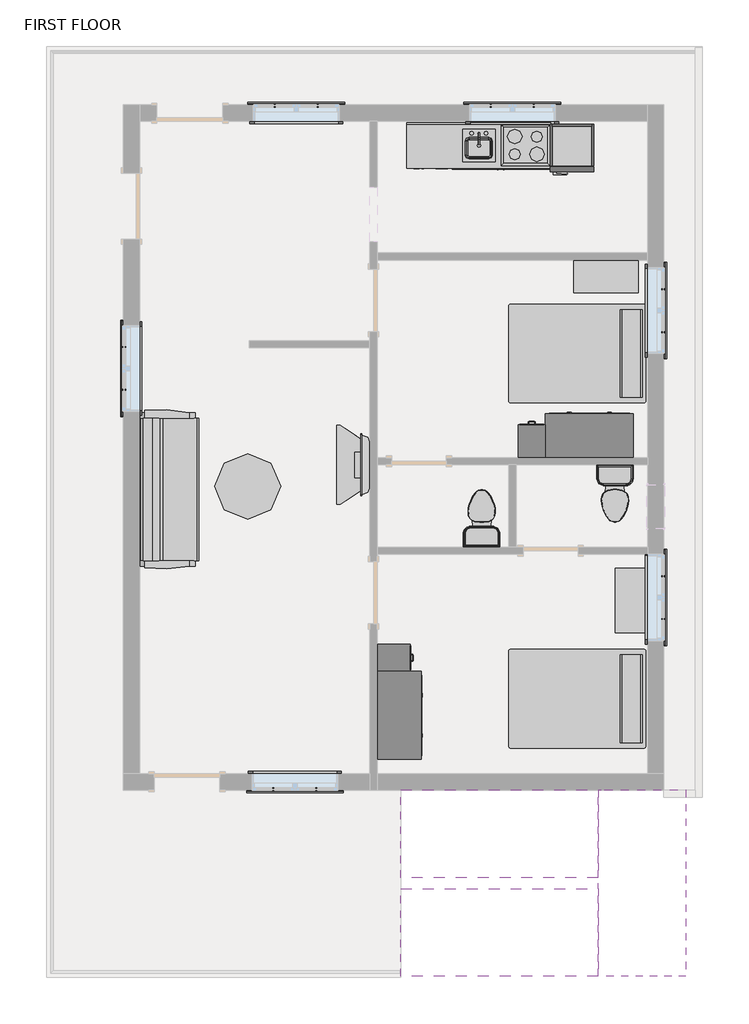
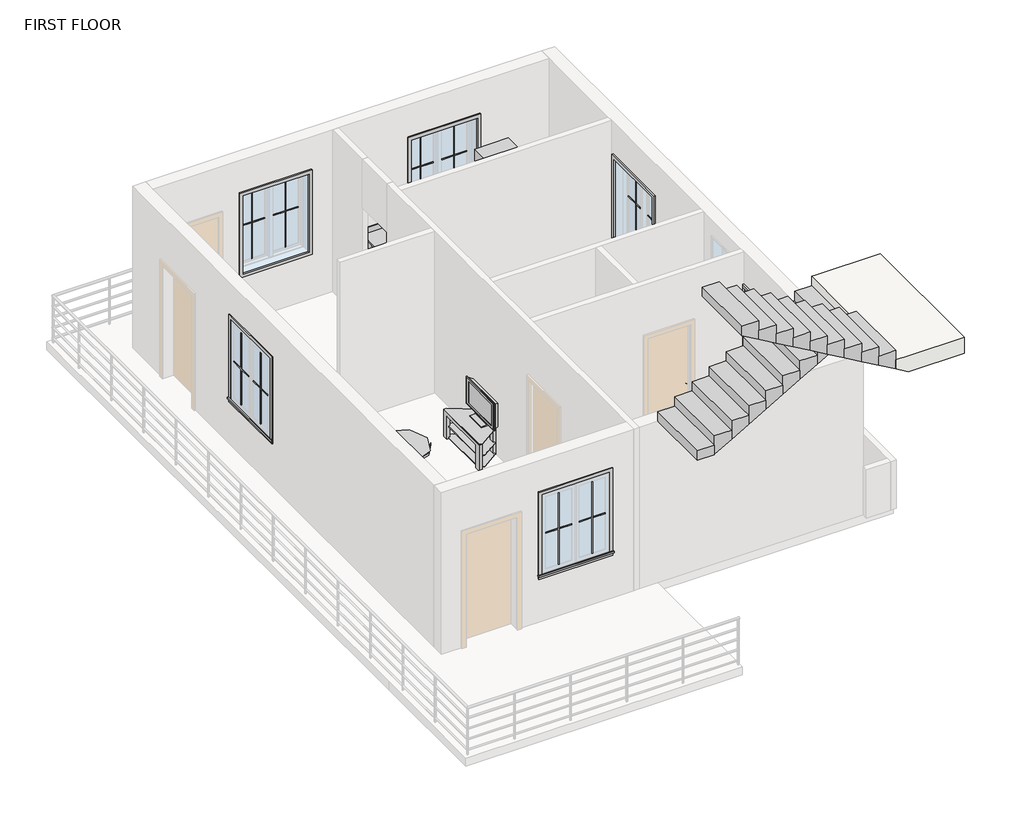
# One storey, part 3 of 3: 28 proxies, 13 furniture elements, 3 flow terminals, 2 stair flights, 1 slab.
"""IFC4 building model written with IfcOpenShell, lengths in millimetres."""

from ifc_helpers import new_model, si_unit, origin, place, context, project, spatial, faceted_brep, transform, mapped, element, save
from components import m_cook_top_4_unit2_0615_x_500mm_c91639ce, m_dishwasher_610_x_610_x_875mm_75336c20, m_kitchenette_medium_m_kitchenette_medium_71e50c56, m_muntin_pattern_2x2_m_muntin_pattern_2x2_d4676b39, m_muntin_pattern_2x2_m_muntin_pattern_2x2_dce6eb8c, m_refrigerator_600_x_660mm_0a899b9c, m_trim_window_exterior_flat_with_sill_a970d7bf, m_trim_window_interior_flat_picture_frame_5bf35ee4, m_sink_kitchen_island_450_x_450mm_f6c2c534, m_toilet_domestic_3d_m_toilet_domestic_3d_ba6479b0, m_toilet_domestic_3d_m_toilet_domestic_3d_1a010dbe, furniture_dc210597, furniture_0810mm_51289c3c, m_bed_standard_1372_x_1905mm_double_64e02cd7, m_cabinet_file_5_drawer_0380_x_0457mm_21dee09a, m_counter_top_w_sink_hole_600mm_depth_2c7d9717, m_dresser_1220_x_1830_x_0610mm_75a9f440, m_furniture_system_storage_cabinet_2_vertical_file_900_x_450_def3fd80, m_sofa_pensi_2134mm_538a523a, m_table_dining_round_0915mm_diameter_394c0b6d

model = new_model("IFC4")

# Units and contexts
model_context = context("Model", 3, world=origin())
ifc_project = project(units=[si_unit("LENGTHUNIT", "METRE", prefix="MILLI")], contexts=[model_context])

# Site, building, storey
site = spatial("IfcSite", under=ifc_project)
building = spatial("IfcBuilding", under=site)
storey = spatial("IfcBuildingStorey", under=building, Name="FIRST FLOOR", Elevation=3200.4)

# Proxies
placement = place(None, origin())
m_cook_top_4_unit2_0615_x_500mm_shape = m_cook_top_4_unit2_0615_x_500mm_c91639ce(model_context)
element("IfcBuildingElementProxy", 1, Name="M_Cook Top-4 Unit2 : 0615 x 500mm", ObjectType="M_Cook Top-4 Unit2 : 0615 x 500mm", at=placement, inside=storey, context=model_context, shape_type="MappedRepresentation", body=[
    mapped(m_cook_top_4_unit2_0615_x_500mm_shape, transform((1952.0701854, 4546.4851347, 3215.4), x_axis=(-1.0, 0.0, 0.0), y_axis=(0.0, -1.0, 0.0), z_axis=(0.0, 0.0, 1.0))),
])
m_dishwasher_610_x_610_x_875mm_shape = m_dishwasher_610_x_610_x_875mm_75336c20(model_context)
element("IfcBuildingElementProxy", 2, Name="M_Dishwasher : 610 x 610 x 875mm", ObjectType="M_Dishwasher : 610 x 610 x 875mm", at=placement, inside=storey, context=model_context, shape_type="MappedRepresentation", body=[
    mapped(m_dishwasher_610_x_610_x_875mm_shape, transform((987.0876539, 4289.8355699, 3200.4), x_axis=(-1.0, 0.0, 0.0), y_axis=(0.0, -1.0, 0.0), z_axis=(0.0, 0.0, 1.0))),
])
m_kitchenette_medium_m_kitchenette_medium_shape = m_kitchenette_medium_m_kitchenette_medium_71e50c56(model_context)
element("IfcBuildingElementProxy", 3, Name="M_Kitchenette - Medium : M_Kitchenette - Medium", ObjectType="M_Kitchenette - Medium : M_Kitchenette - Medium", at=placement, inside=storey, context=model_context, shape_type="MappedRepresentation", body=[
    mapped(m_kitchenette_medium_m_kitchenette_medium_shape, transform((1623.3078903, 4861.4851347, 3200.4), x_axis=(-1.0, 0.0, 0.0), y_axis=(0.0, -1.0, 0.0), z_axis=(0.0, 0.0, 1.0))),
])
m_muntin_pattern_2x2_m_muntin_pattern_2x2_shape = m_muntin_pattern_2x2_m_muntin_pattern_2x2_d4676b39(model_context)
element("IfcBuildingElementProxy", 4, Name="M_Muntin Pattern_2x2 : M_Muntin Pattern_2x2", ObjectType="M_Muntin Pattern_2x2 : M_Muntin Pattern_2x2", at=placement, inside=storey, context=model_context, shape_type="MappedRepresentation", body=[
    mapped(m_muntin_pattern_2x2_m_muntin_pattern_2x2_shape, transform((1466.9330952, 5099.6101347, 4170.25), x_axis=(1.0, 0.0, 0.0), y_axis=(0.0, 1.0, 0.0), z_axis=(0.0, 0.0, 1.0))),
])
element("IfcBuildingElementProxy", 5, Name="M_Muntin Pattern_2x2 : M_Muntin Pattern_2x2", ObjectType="M_Muntin Pattern_2x2 : M_Muntin Pattern_2x2", at=placement, inside=storey, context=model_context, shape_type="MappedRepresentation", body=[
    mapped(m_muntin_pattern_2x2_m_muntin_pattern_2x2_shape, transform((3864.0205952, 2548.5476347, 4170.25), x_axis=(0.0, -1.0, 0.0), y_axis=(1.0, 0.0, 0.0), z_axis=(0.0, 0.0, 1.0))),
])
element("IfcBuildingElementProxy", 6, Name="M_Muntin Pattern_2x2 : M_Muntin Pattern_2x2", ObjectType="M_Muntin Pattern_2x2 : M_Muntin Pattern_2x2", at=placement, inside=storey, context=model_context, shape_type="MappedRepresentation", body=[
    mapped(m_muntin_pattern_2x2_m_muntin_pattern_2x2_shape, transform((3864.0205952, -1440.8523653, 4170.25), x_axis=(0.0, -1.0, 0.0), y_axis=(1.0, 0.0, 0.0), z_axis=(0.0, 0.0, 1.0))),
])
element("IfcBuildingElementProxy", 7, Name="M_Muntin Pattern_2x2 : M_Muntin Pattern_2x2", ObjectType="M_Muntin Pattern_2x2 : M_Muntin Pattern_2x2", at=placement, inside=storey, context=model_context, shape_type="MappedRepresentation", body=[
    mapped(m_muntin_pattern_2x2_m_muntin_pattern_2x2_shape, transform((-3635.3294048, 1147.1226347, 4170.25), x_axis=(0.0, 1.0, 0.0), y_axis=(-1.0, 0.0, 0.0), z_axis=(0.0, 0.0, 1.0))),
])
element("IfcBuildingElementProxy", 8, Name="M_Muntin Pattern_2x2 : M_Muntin Pattern_2x2", ObjectType="M_Muntin Pattern_2x2 : M_Muntin Pattern_2x2", at=placement, inside=storey, context=model_context, shape_type="MappedRepresentation", body=[
    mapped(m_muntin_pattern_2x2_m_muntin_pattern_2x2_shape, transform((-1536.9669048, 5099.6101347, 4170.25), x_axis=(1.0, 0.0, 0.0), y_axis=(0.0, 1.0, 0.0), z_axis=(0.0, 0.0, 1.0))),
])
element("IfcBuildingElementProxy", 9, Name="M_Muntin Pattern_2x2 : M_Muntin Pattern_2x2", ObjectType="M_Muntin Pattern_2x2 : M_Muntin Pattern_2x2", at=placement, inside=storey, context=model_context, shape_type="MappedRepresentation", body=[
    mapped(m_muntin_pattern_2x2_m_muntin_pattern_2x2_shape, transform((-960.1419048, -4406.3398653, 4170.25), x_axis=(-1.0, 0.0, 0.0), y_axis=(0.0, -1.0, 0.0), z_axis=(0.0, 0.0, 1.0))),
])
m_muntin_pattern_2x2_m_muntin_pattern_2x2_2_shape = m_muntin_pattern_2x2_m_muntin_pattern_2x2_dce6eb8c(model_context)
element("IfcBuildingElementProxy", 10, Name="M_Muntin Pattern_2x2 : M_Muntin Pattern_2x2", ObjectType="M_Muntin Pattern_2x2 : M_Muntin Pattern_2x2", at=placement, inside=storey, context=model_context, shape_type="MappedRepresentation", body=[
    mapped(m_muntin_pattern_2x2_m_muntin_pattern_2x2_2_shape, transform((2063.7580952, 5099.6101347, 4170.25), x_axis=(-1.0, 0.0, 0.0), y_axis=(0.0, -1.0, 0.0), z_axis=(0.0, 0.0, 1.0))),
])
element("IfcBuildingElementProxy", 11, Name="M_Muntin Pattern_2x2 : M_Muntin Pattern_2x2", ObjectType="M_Muntin Pattern_2x2 : M_Muntin Pattern_2x2", at=placement, inside=storey, context=model_context, shape_type="MappedRepresentation", body=[
    mapped(m_muntin_pattern_2x2_m_muntin_pattern_2x2_2_shape, transform((3864.0205952, 1951.7226347, 4170.25), x_axis=(0.0, 1.0, 0.0), y_axis=(-1.0, 0.0, 0.0), z_axis=(0.0, 0.0, 1.0))),
])
element("IfcBuildingElementProxy", 12, Name="M_Muntin Pattern_2x2 : M_Muntin Pattern_2x2", ObjectType="M_Muntin Pattern_2x2 : M_Muntin Pattern_2x2", at=placement, inside=storey, context=model_context, shape_type="MappedRepresentation", body=[
    mapped(m_muntin_pattern_2x2_m_muntin_pattern_2x2_2_shape, transform((3864.0205952, -2037.6773653, 4170.25), x_axis=(0.0, 1.0, 0.0), y_axis=(-1.0, 0.0, 0.0), z_axis=(0.0, 0.0, 1.0))),
])
element("IfcBuildingElementProxy", 13, Name="M_Muntin Pattern_2x2 : M_Muntin Pattern_2x2", ObjectType="M_Muntin Pattern_2x2 : M_Muntin Pattern_2x2", at=placement, inside=storey, context=model_context, shape_type="MappedRepresentation", body=[
    mapped(m_muntin_pattern_2x2_m_muntin_pattern_2x2_2_shape, transform((-3635.3294048, 1743.9476347, 4170.25), x_axis=(0.0, -1.0, 0.0), y_axis=(1.0, 0.0, 0.0), z_axis=(0.0, 0.0, 1.0))),
])
element("IfcBuildingElementProxy", 14, Name="M_Muntin Pattern_2x2 : M_Muntin Pattern_2x2", ObjectType="M_Muntin Pattern_2x2 : M_Muntin Pattern_2x2", at=placement, inside=storey, context=model_context, shape_type="MappedRepresentation", body=[
    mapped(m_muntin_pattern_2x2_m_muntin_pattern_2x2_2_shape, transform((-940.1419048, 5099.6101347, 4170.25), x_axis=(-1.0, 0.0, 0.0), y_axis=(0.0, -1.0, 0.0), z_axis=(0.0, 0.0, 1.0))),
])
element("IfcBuildingElementProxy", 15, Name="M_Muntin Pattern_2x2 : M_Muntin Pattern_2x2", ObjectType="M_Muntin Pattern_2x2 : M_Muntin Pattern_2x2", at=placement, inside=storey, context=model_context, shape_type="MappedRepresentation", body=[
    mapped(m_muntin_pattern_2x2_m_muntin_pattern_2x2_2_shape, transform((-1556.9669048, -4406.3398653, 4170.25), x_axis=(1.0, 0.0, 0.0), y_axis=(0.0, 1.0, 0.0), z_axis=(0.0, 0.0, 1.0))),
])
m_refrigerator_600_x_660mm_shape = m_refrigerator_600_x_660mm_0a899b9c(model_context)
element("IfcBuildingElementProxy", 16, Name="M_Refrigerator : 600 x 660mm", ObjectType="M_Refrigerator : 600 x 660mm", at=placement, inside=storey, context=model_context, shape_type="MappedRepresentation", body=[
    mapped(m_refrigerator_600_x_660mm_shape, transform((2541.7251841, 4544.3679413, 3200.4), x_axis=(-1.0, 0.0, 0.0), y_axis=(0.0, -1.0, 0.0), z_axis=(0.0, 0.0, 1.0))),
])
m_trim_window_exterior_flat_with_sill_shape = m_trim_window_exterior_flat_with_sill_a970d7bf(model_context)
element("IfcBuildingElementProxy", 17, Name="M_Trim-Window-Exterior-Flat : with Sill", ObjectType="M_Trim-Window-Exterior-Flat : with Sill", at=placement, inside=storey, context=model_context, shape_type="MappedRepresentation", body=[
    mapped(m_trim_window_exterior_flat_with_sill_shape, transform((1765.3455952, 5109.1351347, 5600.4), x_axis=(-1.0, 0.0, 0.0), y_axis=(0.0, 0.0, 1.0), z_axis=(0.0, 1.0, 0.0))),
])
element("IfcBuildingElementProxy", 18, Name="M_Trim-Window-Exterior-Flat : with Sill", ObjectType="M_Trim-Window-Exterior-Flat : with Sill", at=placement, inside=storey, context=model_context, shape_type="MappedRepresentation", body=[
    mapped(m_trim_window_exterior_flat_with_sill_shape, transform((3873.5455952, 2250.1351347, 5600.4), x_axis=(0.0, 1.0, 0.0), y_axis=(0.0, 0.0, 1.0), z_axis=(1.0, 0.0, 0.0))),
])
element("IfcBuildingElementProxy", 19, Name="M_Trim-Window-Exterior-Flat : with Sill", ObjectType="M_Trim-Window-Exterior-Flat : with Sill", at=placement, inside=storey, context=model_context, shape_type="MappedRepresentation", body=[
    mapped(m_trim_window_exterior_flat_with_sill_shape, transform((3873.5455952, -1739.2648653, 5600.4), x_axis=(0.0, 1.0, 0.0), y_axis=(0.0, 0.0, 1.0), z_axis=(1.0, 0.0, 0.0))),
])
element("IfcBuildingElementProxy", 20, Name="M_Trim-Window-Exterior-Flat : with Sill", ObjectType="M_Trim-Window-Exterior-Flat : with Sill", at=placement, inside=storey, context=model_context, shape_type="MappedRepresentation", body=[
    mapped(m_trim_window_exterior_flat_with_sill_shape, transform((-3644.8544048, 1445.5351347, 5600.4), x_axis=(0.0, -1.0, 0.0), y_axis=(0.0, 0.0, 1.0), z_axis=(-1.0, 0.0, 0.0))),
])
element("IfcBuildingElementProxy", 21, Name="M_Trim-Window-Exterior-Flat : with Sill", ObjectType="M_Trim-Window-Exterior-Flat : with Sill", at=placement, inside=storey, context=model_context, shape_type="MappedRepresentation", body=[
    mapped(m_trim_window_exterior_flat_with_sill_shape, transform((-1238.5544048, 5109.1351347, 5600.4), x_axis=(-1.0, 0.0, 0.0), y_axis=(0.0, 0.0, 1.0), z_axis=(0.0, 1.0, 0.0))),
])
element("IfcBuildingElementProxy", 22, Name="M_Trim-Window-Exterior-Flat : with Sill", ObjectType="M_Trim-Window-Exterior-Flat : with Sill", at=placement, inside=storey, context=model_context, shape_type="MappedRepresentation", body=[
    mapped(m_trim_window_exterior_flat_with_sill_shape, transform((-1258.5544048, -4415.8648653, 5600.4), x_axis=(1.0, 0.0, 0.0), y_axis=(0.0, 0.0, 1.0), z_axis=(0.0, -1.0, 0.0))),
])
m_trim_window_interior_flat_picture_frame_shape = m_trim_window_interior_flat_picture_frame_5bf35ee4(model_context)
element("IfcBuildingElementProxy", 23, Name="M_Trim-Window-Interior-Flat : Picture Frame", ObjectType="M_Trim-Window-Interior-Flat : Picture Frame", at=placement, inside=storey, context=model_context, shape_type="MappedRepresentation", body=[
    mapped(m_trim_window_interior_flat_picture_frame_shape, transform((1765.3455952, 4880.5351347, 5600.4), x_axis=(1.0, 0.0, 0.0), y_axis=(0.0, 0.0, 1.0), z_axis=(0.0, -1.0, 0.0))),
])
element("IfcBuildingElementProxy", 24, Name="M_Trim-Window-Interior-Flat : Picture Frame", ObjectType="M_Trim-Window-Interior-Flat : Picture Frame", at=placement, inside=storey, context=model_context, shape_type="MappedRepresentation", body=[
    mapped(m_trim_window_interior_flat_picture_frame_shape, transform((3644.9455952, 2250.1351347, 5600.4), x_axis=(0.0, -1.0, 0.0), y_axis=(0.0, 0.0, 1.0), z_axis=(-1.0, 0.0, 0.0))),
])
element("IfcBuildingElementProxy", 25, Name="M_Trim-Window-Interior-Flat : Picture Frame", ObjectType="M_Trim-Window-Interior-Flat : Picture Frame", at=placement, inside=storey, context=model_context, shape_type="MappedRepresentation", body=[
    mapped(m_trim_window_interior_flat_picture_frame_shape, transform((3644.9455952, -1739.2648653, 5600.4), x_axis=(0.0, -1.0, 0.0), y_axis=(0.0, 0.0, 1.0), z_axis=(-1.0, 0.0, 0.0))),
])
element("IfcBuildingElementProxy", 26, Name="M_Trim-Window-Interior-Flat : Picture Frame", ObjectType="M_Trim-Window-Interior-Flat : Picture Frame", at=placement, inside=storey, context=model_context, shape_type="MappedRepresentation", body=[
    mapped(m_trim_window_interior_flat_picture_frame_shape, transform((-3416.2544048, 1445.5351347, 5600.4), x_axis=(0.0, 1.0, 0.0), y_axis=(0.0, 0.0, 1.0), z_axis=(1.0, 0.0, 0.0))),
])
element("IfcBuildingElementProxy", 27, Name="M_Trim-Window-Interior-Flat : Picture Frame", ObjectType="M_Trim-Window-Interior-Flat : Picture Frame", at=placement, inside=storey, context=model_context, shape_type="MappedRepresentation", body=[
    mapped(m_trim_window_interior_flat_picture_frame_shape, transform((-1238.5544048, 4880.5351347, 5600.4), x_axis=(1.0, 0.0, 0.0), y_axis=(0.0, 0.0, 1.0), z_axis=(0.0, -1.0, 0.0))),
])
element("IfcBuildingElementProxy", 28, Name="M_Trim-Window-Interior-Flat : Picture Frame", ObjectType="M_Trim-Window-Interior-Flat : Picture Frame", at=placement, inside=storey, context=model_context, shape_type="MappedRepresentation", body=[
    mapped(m_trim_window_interior_flat_picture_frame_shape, transform((-1258.5544048, -4187.2648653, 5600.4), x_axis=(-1.0, 0.0, 0.0), y_axis=(0.0, 0.0, 1.0), z_axis=(0.0, 1.0, 0.0))),
])

# Flow terminals
m_sink_kitchen_island_450_x_450mm_shape = m_sink_kitchen_island_450_x_450mm_f6c2c534(model_context)
element("IfcFlowTerminal", 29, ObjectType="M_Sink Kitchen-Island : 450 x 450mm", at=placement, inside=storey, context=model_context, shape_type="MappedRepresentation", body=[
    mapped(m_sink_kitchen_island_450_x_450mm_shape, transform((1315.2594259, 4546.0397336, 3215.4), x_axis=(-1.0, 0.0, 0.0), y_axis=(0.0, -1.0, 0.0), z_axis=(0.0, 0.0, 1.0))),
])
m_toilet_domestic_3d_m_toilet_domestic_3d_shape = m_toilet_domestic_3d_m_toilet_domestic_3d_ba6479b0(model_context)
m_toilet_domestic_3d_m_toilet_domestic_3d_2_shape = m_toilet_domestic_3d_m_toilet_domestic_3d_1a010dbe(model_context)
element("IfcFlowTerminal", 30, ObjectType="M_Toilet-Domestic-3D : M_Toilet-Domestic-3D", at=placement, inside=storey, context=model_context, shape_type="MappedRepresentation", body=[
    mapped(m_toilet_domestic_3d_m_toilet_domestic_3d_shape, transform((3191.5495678, -389.3608926, 3200.4), x_axis=(1.0, 0.0, 0.0), y_axis=(0.0, 1.0, 0.0), z_axis=(0.0, 0.0, 1.0))),
    mapped(m_toilet_domestic_3d_m_toilet_domestic_3d_2_shape, transform((3191.5495678, -389.3608926, 3200.4), x_axis=(1.0, 0.0, 0.0), y_axis=(0.0, 1.0, 0.0), z_axis=(0.0, 0.0, 1.0))),
])
element("IfcFlowTerminal", 31, ObjectType="M_Toilet-Domestic-3D : M_Toilet-Domestic-3D", at=placement, inside=storey, context=model_context, shape_type="MappedRepresentation", body=[
    mapped(m_toilet_domestic_3d_m_toilet_domestic_3d_shape, transform((1339.1416225, -542.9688379, 3200.4), x_axis=(-1.0, 0.0, 0.0), y_axis=(0.0, -1.0, 0.0), z_axis=(0.0, 0.0, 1.0))),
    mapped(m_toilet_domestic_3d_m_toilet_domestic_3d_2_shape, transform((1339.1416225, -542.9688379, 3200.4), x_axis=(-1.0, 0.0, 0.0), y_axis=(0.0, -1.0, 0.0), z_axis=(0.0, 0.0, 1.0))),
])

# Furniture
furniture_shape = furniture_dc210597(model_context)
element("IfcFurniture", 32, at=placement, inside=storey, context=model_context, shape_type="MappedRepresentation", body=[
    mapped(furniture_shape, transform((-215.8544048, 230.5231368, 3200.4), x_axis=(0.0, -1.0, 0.0), y_axis=(1.0, 0.0, 0.0), z_axis=(0.0, 0.0, 1.0))),
])
furniture_0810mm_shape = furniture_0810mm_51289c3c(model_context)
element("IfcFurniture", 33, ObjectType="0810mm", at=placement, inside=storey, context=model_context, shape_type="MappedRepresentation", body=[
    mapped(furniture_0810mm_shape, transform((-274.3930285, 101.3906206, 3710.4), x_axis=(0.0, -1.0, 0.0), y_axis=(1.0, 0.0, 0.0), z_axis=(0.0, 0.0, 1.0))),
])
m_bed_standard_1372_x_1905mm_double_shape = m_bed_standard_1372_x_1905mm_double_64e02cd7(model_context)
element("IfcFurniture", 34, ObjectType="M_Bed-Standard : 1372 x 1905mm - Double", at=placement, inside=storey, context=model_context, shape_type="MappedRepresentation", body=[
    mapped(m_bed_standard_1372_x_1905mm_double_shape, transform((2712.6406772, -2874.5763407, 3200.4), x_axis=(0.0, -1.0, 0.0), y_axis=(1.0, 0.0, 0.0), z_axis=(0.0, 0.0, 1.0))),
])
element("IfcFurniture", 35, ObjectType="M_Bed-Standard : 1372 x 1905mm - Double", at=placement, inside=storey, context=model_context, shape_type="MappedRepresentation", body=[
    mapped(m_bed_standard_1372_x_1905mm_double_shape, transform((2712.6406772, 1925.4236593, 3200.4), x_axis=(0.0, -1.0, 0.0), y_axis=(1.0, 0.0, 0.0), z_axis=(0.0, 0.0, 1.0))),
])
m_cabinet_file_5_drawer_0380_x_0457mm_shape = m_cabinet_file_5_drawer_0380_x_0457mm_21dee09a(model_context)
element("IfcFurniture", 36, ObjectType="M_Cabinet-File 5 Drawer : 0380 x 0457mm", at=placement, inside=storey, context=model_context, shape_type="MappedRepresentation", body=[
    mapped(m_cabinet_file_5_drawer_0380_x_0457mm_shape, transform((-27.8887049, -2449.3684182, 3200.4), x_axis=(0.0, 1.0, 0.0), y_axis=(-1.0, 0.0, 0.0), z_axis=(0.0, 0.0, 1.0))),
])
element("IfcFurniture", 37, ObjectType="M_Cabinet-File 5 Drawer : 0380 x 0457mm", at=placement, inside=storey, context=model_context, shape_type="MappedRepresentation", body=[
    mapped(m_cabinet_file_5_drawer_0380_x_0457mm_shape, transform((1907.0491482, 293.3008346, 3200.4), x_axis=(-1.0, 0.0, 0.0), y_axis=(0.0, -1.0, 0.0), z_axis=(0.0, 0.0, 1.0))),
])
m_counter_top_w_sink_hole_600mm_depth_shape = m_counter_top_w_sink_hole_600mm_depth_2c7d9717(model_context)
element("IfcFurniture", 38, ObjectType="M_Counter Top w Sink Hole : 600mm Depth", at=placement, inside=storey, context=model_context, shape_type="MappedRepresentation", body=[
    mapped(m_counter_top_w_sink_hole_600mm_depth_shape, transform((1099.1078903, 4861.4851347, 3215.4), x_axis=(-1.0, 0.0, 0.0), y_axis=(0.0, -1.0, 0.0), z_axis=(0.0, 0.0, 1.0))),
])
m_dresser_1220_x_1830_x_0610mm_shape = m_dresser_1220_x_1830_x_0610mm_75a9f440(model_context)
element("IfcFurniture", 39, ObjectType="M_Dresser : 1220 x 1830 x 0610mm", at=placement, inside=storey, context=model_context, shape_type="MappedRepresentation", body=[
    mapped(m_dresser_1220_x_1830_x_0610mm_shape, transform((2565.7523354, 148.7721806, 3200.4), x_axis=(-1.0, 0.0, 0.0), y_axis=(0.0, -1.0, 0.0), z_axis=(0.0, 0.0, 1.0))),
])
element("IfcFurniture", 40, ObjectType="M_Dresser : 1220 x 1830 x 0610mm", at=placement, inside=storey, context=model_context, shape_type="MappedRepresentation", body=[
    mapped(m_dresser_1220_x_1830_x_0610mm_shape, transform((-172.4173589, -3108.0716054, 3200.4), x_axis=(0.0, 1.0, 0.0), y_axis=(-1.0, 0.0, 0.0), z_axis=(0.0, 0.0, 1.0))),
])
m_furniture_system_storage_cabinet_2_vertical_file_900_x_450_shape = m_furniture_system_storage_cabinet_2_vertical_file_900_x_450_def3fd80(model_context)
element("IfcFurniture", 41, ObjectType="M_Furniture_System-Storage-Cabinet-2_Vertical_File : 900 x 450 x 650mm", at=placement, inside=storey, context=model_context, shape_type="MappedRepresentation", body=[
    mapped(m_furniture_system_storage_cabinet_2_vertical_file_900_x_450_shape, transform((3066.1455952, 2500.1351347, 3200.4), x_axis=(1.0, 0.0, 0.0), y_axis=(0.0, 1.0, 0.0), z_axis=(0.0, 0.0, 1.0))),
])
element("IfcFurniture", 42, ObjectType="M_Furniture_System-Storage-Cabinet-2_Vertical_File : 900 x 450 x 650mm", at=placement, inside=storey, context=model_context, shape_type="MappedRepresentation", body=[
    mapped(m_furniture_system_storage_cabinet_2_vertical_file_900_x_450_shape, transform((3194.9455952, -1781.4648653, 3200.4), x_axis=(0.0, -1.0, 0.0), y_axis=(1.0, 0.0, 0.0), z_axis=(0.0, 0.0, 1.0))),
])
m_sofa_pensi_2134mm_shape = m_sofa_pensi_2134mm_538a523a(model_context)
element("IfcFurniture", 43, ObjectType="M_Sofa-Pensi : 2134mm", at=placement, inside=storey, context=model_context, shape_type="MappedRepresentation", body=[
    mapped(m_sofa_pensi_2134mm_shape, transform((-2738.7445687, -514.3711153, 3200.4), x_axis=(0.0, 1.0, 0.0), y_axis=(-1.0, 0.0, 0.0), z_axis=(0.0, 0.0, 1.0))),
])
m_table_dining_round_0915mm_diameter_shape = m_table_dining_round_0915mm_diameter_394c0b6d(model_context)
element("IfcFurniture", 44, ObjectType="M_Table-Dining Round : 0915mm Diameter", at=placement, inside=storey, context=model_context, shape_type="MappedRepresentation", body=[
    mapped(m_table_dining_round_0915mm_diameter_shape, transform((-2019.536372, -9.7861767, 3200.4), x_axis=(1.0, 0.0, 0.0), y_axis=(0.0, 1.0, 0.0), z_axis=(0.0, 0.0, 1.0))),
])

# Slab
element("IfcSlab", 45, ObjectType="300mm Thickness", at=placement, inside=storey, context=model_context, shape_type="Brep", body=[
    faceted_brep([(2959.1455952, -4415.8648653, 8013.0315789), (2959.1455952, -5635.0648653, 8013.0315789), (2959.1455952, -5787.4648653, 8013.0315789), (2959.1455952, -7006.6648653, 8013.0315789), (3177.9478897, -7006.6648653, 8013.0315789), (4178.3455952, -7006.6648653, 8013.0315789), (4178.3455952, -4415.8648653, 8013.0315789), (3045.1433006, -4415.8648653, 8013.0315789), (2959.1455952, -4415.8648653, 7836.5684211), (2959.1455952, -4415.8648653, 7663.2434337), (2959.1455952, -5635.0648653, 7663.2434337), (2959.1455952, -5635.0648653, 7713.0315789), (2959.1455952, -5787.4648653, 7713.0315789), (2959.1455952, -5787.4648653, 7839.7065916), (2959.1455952, -7006.6648653, 7839.7065916), (3177.9478897, -7006.6648653, 7713.0315789), (4178.3455952, -7006.6648653, 7713.0315789), (4178.3455952, -4415.8648653, 7713.0315789), (3045.1433006, -4415.8648653, 7713.0315789), (3177.9478897, -5787.4648653, 7713.0315789), (3045.1433006, -5635.0648653, 7713.0315789)], [[[0, 1, 2, 3, 4, 5, 6, 7]], [[1, 0, 8, 9, 10, 11]], [[2, 1, 11, 12, 13]], [[3, 2, 13, 14]], [[3, 14, 15, 16, 5, 4]], [[6, 5, 16, 17]], [[9, 8, 0, 7, 6, 17, 18]], [[19, 12, 11, 20, 18, 17, 16, 15]], [[12, 19, 13]], [[18, 20, 10, 9]], [[20, 11, 10]], [[19, 15, 14, 13]]]),
])

# Stair flights
element("IfcStairFlight", 46, ObjectType="150mm Depth", at=placement, inside=storey, context=model_context, shape_type="Brep", body=[
    faceted_brep([(520.7455952, -4415.8648653, 6424.8631579), (215.9455952, -4415.8648653, 6424.8631579), (215.9455952, -5635.0648653, 6424.8631579), (520.7455952, -5635.0648653, 6424.8631579), (520.7455952, -4415.8648653, 6251.5381705), (515.3251188, -4415.8648653, 6248.4), (215.9455952, -4415.8648653, 6248.4), (215.9455952, -5635.0648653, 6248.4), (515.3251188, -5635.0648653, 6248.4), (520.7455952, -5635.0648653, 6251.5381705), (825.5455952, -4415.8648653, 6601.3263158), (520.7455952, -4415.8648653, 6601.3263158), (520.7455952, -5635.0648653, 6601.3263158), (825.5455952, -5635.0648653, 6601.3263158), (825.5455952, -4415.8648653, 6428.0013284), (825.5455952, -5635.0648653, 6428.0013284), (1130.3455952, -4415.8648653, 6777.7894737), (825.5455952, -4415.8648653, 6777.7894737), (825.5455952, -5635.0648653, 6777.7894737), (1130.3455952, -5635.0648653, 6777.7894737), (1130.3455952, -4415.8648653, 6604.4644863), (1130.3455952, -5635.0648653, 6604.4644863), (1435.1455952, -4415.8648653, 6954.2526316), (1130.3455952, -4415.8648653, 6954.2526316), (1130.3455952, -5635.0648653, 6954.2526316), (1435.1455952, -5635.0648653, 6954.2526316), (1435.1455952, -4415.8648653, 6780.9276442), (1435.1455952, -5635.0648653, 6780.9276442), (1739.9455952, -4415.8648653, 7130.7157895), (1435.1455952, -4415.8648653, 7130.7157895), (1435.1455952, -5635.0648653, 7130.7157895), (1739.9455952, -5635.0648653, 7130.7157895), (1739.9455952, -4415.8648653, 6957.3908021), (1739.9455952, -5635.0648653, 6957.3908021), (2044.7455952, -4415.8648653, 7307.1789474), (1739.9455952, -4415.8648653, 7307.1789474), (1739.9455952, -5635.0648653, 7307.1789474), (2044.7455952, -5635.0648653, 7307.1789474), (2044.7455952, -4415.8648653, 7133.85396), (2044.7455952, -5635.0648653, 7133.85396), (2349.5455952, -4415.8648653, 7483.6421053), (2044.7455952, -4415.8648653, 7483.6421053), (2044.7455952, -5635.0648653, 7483.6421053), (2349.5455952, -5635.0648653, 7483.6421053), (2349.5455952, -4415.8648653, 7310.3171179), (2349.5455952, -5635.0648653, 7310.3171179), (2654.3455952, -4415.8648653, 7660.1052632), (2349.5455952, -4415.8648653, 7660.1052632), (2349.5455952, -5635.0648653, 7660.1052632), (2654.3455952, -5635.0648653, 7660.1052632), (2654.3455952, -4415.8648653, 7486.7802758), (2654.3455952, -5635.0648653, 7486.7802758), (2959.1455952, -4415.8648653, 7836.5684211), (2654.3455952, -4415.8648653, 7836.5684211), (2654.3455952, -5635.0648653, 7836.5684211), (2959.1455952, -5635.0648653, 7836.5684211), (2959.1455952, -4415.8648653, 7663.2434337), (2959.1455952, -5635.0648653, 7663.2434337), (2959.1455952, -5635.0648653, 7713.0315789)], [[[0, 1, 2, 3]], [[1, 0, 4, 5, 6]], [[2, 1, 6, 7]], [[3, 2, 7, 8, 9]], [[10, 11, 12, 13]], [[11, 10, 14, 4, 0]], [[0, 3, 12, 11]], [[13, 12, 3, 9, 15]], [[16, 17, 18, 19]], [[17, 16, 20, 14, 10]], [[10, 13, 18, 17]], [[19, 18, 13, 15, 21]], [[22, 23, 24, 25]], [[23, 22, 26, 20, 16]], [[16, 19, 24, 23]], [[25, 24, 19, 21, 27]], [[28, 29, 30, 31]], [[29, 28, 32, 26, 22]], [[22, 25, 30, 29]], [[31, 30, 25, 27, 33]], [[34, 35, 36, 37]], [[35, 34, 38, 32, 28]], [[28, 31, 36, 35]], [[37, 36, 31, 33, 39]], [[40, 41, 42, 43]], [[41, 40, 44, 38, 34]], [[34, 37, 42, 41]], [[43, 42, 37, 39, 45]], [[46, 47, 48, 49]], [[47, 46, 50, 44, 40]], [[40, 43, 48, 47]], [[49, 48, 43, 45, 51]], [[52, 53, 54, 55]], [[53, 52, 56, 50, 46]], [[46, 49, 54, 53]], [[55, 54, 49, 51, 57, 58]], [[52, 55, 58, 57, 56]], [[7, 6, 5, 8]], [[8, 5, 4, 14, 20, 26, 32, 38, 44, 50, 56, 57, 51, 45, 39, 33, 27, 21, 15, 9]]]),
])
element("IfcStairFlight", 47, ObjectType="150mm Depth", at=placement, inside=storey, context=model_context, shape_type="Brep", body=[
    faceted_brep([(2654.3455952, -7006.6648653, 8189.4947368), (2959.1455952, -7006.6648653, 8189.4947368), (2959.1455952, -5787.4648653, 8189.4947368), (2654.3455952, -5787.4648653, 8189.4947368), (2654.3455952, -7006.6648653, 8016.1697495), (2959.1455952, -7006.6648653, 7839.7065916), (2959.1455952, -7006.6648653, 8013.0315789), (2959.1455952, -5787.4648653, 7839.7065916), (2654.3455952, -5787.4648653, 8016.1697495), (2349.5455952, -7006.6648653, 8365.9578947), (2654.3455952, -7006.6648653, 8365.9578947), (2654.3455952, -5787.4648653, 8365.9578947), (2349.5455952, -5787.4648653, 8365.9578947), (2349.5455952, -7006.6648653, 8192.6329074), (2349.5455952, -5787.4648653, 8192.6329074), (2044.7455952, -7006.6648653, 8542.4210526), (2349.5455952, -7006.6648653, 8542.4210526), (2349.5455952, -5787.4648653, 8542.4210526), (2044.7455952, -5787.4648653, 8542.4210526), (2044.7455952, -7006.6648653, 8369.0960653), (2044.7455952, -5787.4648653, 8369.0960653), (1739.9455952, -7006.6648653, 8718.8842105), (2044.7455952, -7006.6648653, 8718.8842105), (2044.7455952, -5787.4648653, 8718.8842105), (1739.9455952, -5787.4648653, 8718.8842105), (1739.9455952, -7006.6648653, 8545.5592232), (1739.9455952, -5787.4648653, 8545.5592232), (1435.1455952, -7006.6648653, 8895.3473684), (1739.9455952, -7006.6648653, 8895.3473684), (1739.9455952, -5787.4648653, 8895.3473684), (1435.1455952, -5787.4648653, 8895.3473684), (1435.1455952, -7006.6648653, 8722.0223811), (1435.1455952, -5787.4648653, 8722.0223811), (1130.3455952, -7006.6648653, 9071.8105263), (1435.1455952, -7006.6648653, 9071.8105263), (1435.1455952, -5787.4648653, 9071.8105263), (1130.3455952, -5787.4648653, 9071.8105263), (1130.3455952, -7006.6648653, 8898.4855389), (1130.3455952, -5787.4648653, 8898.4855389), (825.5455952, -7006.6648653, 9248.2736842), (1130.3455952, -7006.6648653, 9248.2736842), (1130.3455952, -5787.4648653, 9248.2736842), (825.5455952, -5787.4648653, 9248.2736842), (825.5455952, -7006.6648653, 9074.9486968), (825.5455952, -5787.4648653, 9074.9486968), (520.7455952, -7006.6648653, 9424.7368421), (825.5455952, -7006.6648653, 9424.7368421), (825.5455952, -5787.4648653, 9424.7368421), (520.7455952, -5787.4648653, 9424.7368421), (520.7455952, -7006.6648653, 9251.4118547), (520.7455952, -5787.4648653, 9251.4118547), (215.9455952, -7006.6648653, 9601.2), (520.7455952, -7006.6648653, 9601.2), (520.7455952, -5787.4648653, 9601.2), (215.9455952, -5787.4648653, 9601.2), (215.9455952, -7006.6648653, 9427.8750126), (215.9455952, -5787.4648653, 9427.8750126)], [[[0, 1, 2, 3]], [[1, 0, 4, 5, 6]], [[2, 1, 6, 5, 7]], [[3, 2, 7, 8]], [[9, 10, 11, 12]], [[10, 9, 13, 4, 0]], [[11, 10, 0, 3]], [[12, 11, 3, 8, 14]], [[15, 16, 17, 18]], [[16, 15, 19, 13, 9]], [[17, 16, 9, 12]], [[18, 17, 12, 14, 20]], [[21, 22, 23, 24]], [[22, 21, 25, 19, 15]], [[23, 22, 15, 18]], [[24, 23, 18, 20, 26]], [[27, 28, 29, 30]], [[28, 27, 31, 25, 21]], [[29, 28, 21, 24]], [[30, 29, 24, 26, 32]], [[33, 34, 35, 36]], [[34, 33, 37, 31, 27]], [[35, 34, 27, 30]], [[36, 35, 30, 32, 38]], [[39, 40, 41, 42]], [[40, 39, 43, 37, 33]], [[41, 40, 33, 36]], [[42, 41, 36, 38, 44]], [[45, 46, 47, 48]], [[46, 45, 49, 43, 39]], [[47, 46, 39, 42]], [[48, 47, 42, 44, 50]], [[51, 52, 53, 54]], [[52, 51, 55, 49, 45]], [[53, 52, 45, 48]], [[54, 53, 48, 50, 56]], [[51, 54, 56, 55]], [[5, 4, 13, 19, 25, 31, 37, 43, 49, 55, 56, 50, 44, 38, 32, 26, 20, 14, 8, 7]]]),
])

save(model, "model.ifc")

# Revit data of these elements
# Type "M_Cook Top-4 Unit2 : 0615 x 500mm"
#   Depth = 1.64042 ft
#   Width = 2.017717 ft
#   Burner Material = Steel, Chrome Plated
#   Cooktop Material = Steel, Polished
#   Default Elevation = 0
#   Assembly Code = ""
# Type "M_Dishwasher : 610 x 610 x 875mm"
#   Label = "DW"
#   Depth = 2.001312 ft
#   Height = 2.870735 ft
#   Width = 2.001312 ft
#   Dishwasher Material = Steel, Paint Finish, Ivory, Glossy
#   Panel Face Material = Plastic, Opaque Black
#   Default Elevation = 0
# Type "M_Kitchenette - Medium : M_Kitchenette - Medium"
#   Sink Opening Depth = 1.148294 ft
#   Sink Location To Wall = 0.492126 ft
#   Sink Location = 3.28084 ft
#   Counter Thickness = 0.131234 ft
#   Counter Length = 6.56168 ft
#   Cabinet Width = 4.560367 ft
#   Cabinet Height = 2.870735 ft
#   Cabinet Depth = 2.066929 ft
#   Toe Depth = 0.114829 ft
#   Toe Height = 0.328084 ft
#   Cabinet Material = Cabinets
#   Door/Drawer Material = Cabinets
#   Handle Material = Cabinets - Handles
#   Default Elevation = 0
# Type "M_Muntin Pattern_2x2 : M_Muntin Pattern_2x2"
#   Width [instance default] = 3.937008 ft
#   Thickness = 0.041667 ft
#   Height [instance default] = 3.937008 ft
#   Distance = 0.0625 ft
#   Interior Material [instance default] = none
#   Exterior Material [instance default] = none
#   Default Elevation = 0
# Type "M_Refrigerator : 600 x 660mm"
#   Label = "REF."
#   Depth = 2.165354 ft
#   Height = 6.003937 ft
#   Width = 1.968504 ft
#   Material = Steel, Paint Finish, Ivory, Matte
#   Description = (empty or 0)
#   Default Elevation = 0
# Type "M_Trim-Window-Exterior-Flat : with Sill"
#   Trim Width = 0.19685 ft
#   Trim Thickness_Picture Frame = 0.098425 ft
#   Trim Thickness_with Sill = 0.0625 ft
#   Sill Thickness = 0.098425 ft
#   Opening Width [instance default] = 1.968504 ft
#   Opening Height [instance default] = 2.952756 ft
#   Default Elevation = 3.937008 ft
#   Sill = yes
#   Picture Frame = no
#   Trim Material [instance default] = none
# Type "M_Trim-Window-Interior-Flat : Picture Frame"
#   Trim Thickness_Picture Frame = 0.098425 ft
#   Trim Width = 0.19685 ft
#   Trim Thickness_with Sill = 0.065617 ft
#   Sill Thickness = 0.098425 ft
#   Opening Width [instance default] = 1.968504 ft
#   Opening Height [instance default] = 2.952756 ft
#   Default Elevation = 3.937008 ft
#   Sill = no
#   Picture Frame = yes
#   Trim Material [instance default] = none
# Type "M_Sink Kitchen-Island : 450 x 450mm"
#   Counter Height [instance default] = 2.952756 ft
#   Depth = 1.476378 ft
#   Width = 1.476378 ft
#   Fixture Material = Steel, Polished
#   Sink Material = Steel, Polished
#   Default Elevation = 0
# Type "M_Toilet-Domestic-3D : M_Toilet-Domestic-3D"
#   Bowl/Basin Material = Porcelain, Linen
#   Seat Material = Laminate, Linen, Matte
#   Default Elevation = 0
# Type
#   Depth = 1.509186 ft
#   Width = 3.608924 ft
#   Height = 1.64042 ft
#   Finish = Melamine - Gray
#   Default Elevation = 0
# Type "0810mm"
#   SinAng = 0.001609 ft
#   L = 2.316144 ft
#   H = 1.30295 ft
#   Thickness = 0.360892 ft
#   Diagonal = 2.65748 ft
#   CosAng = 0.002859 ft
#   Stand [instance default] = yes
#   Default Elevation = 0
# Type "M_Bed-Standard : 1372 x 1905mm - Double"
#   Length = 6.25 ft
#   Width = 4.501312 ft
#   Leg Material = Steel, Chrome Plated
#   Mattress Material = Linen, White
#   Default Elevation = 0
# Type "M_Cabinet-File 5 Drawer : 0380 x 0457mm"
#   Depth = 1.499344 ft
#   Height = 5.003281 ft
#   Width = 1.246719 ft
#   Cabinet Material = Steel, Paint Finish, Ivory, Glossy
#   Handle Material = Steel, Chrome Plated
#   Default Elevation = 0
# Type "M_Counter Top w Sink Hole : 600mm Depth"
#   Counter Thickness = 0.131234 ft
#   Depth [instance default] = 2.050525 ft
#   Height = 2.952756 ft
#   Length [instance default] = 8.2021 ft
#   Sink Location [instance default] = 3.937008 ft
#   Sink Location To Wall [instance default] = 0.328084 ft
#   Sink Opening Depth [instance default] = 1.240157 ft
#   Sink Opening Width [instance default] = 1.925853 ft
#   Counter Top Material = none
#   Default Elevation = 0
# Type "M_Dresser : 1220 x 1830 x 0610mm"
#   Depth = 2.001312 ft
#   Height = 6.003937 ft
#   Width = 4.002625 ft
#   Dresser Material = Laminate - Ivory, Glossy
#   Drawer Material = Laminate, Ivory, Matte
#   Knob Material = Cherry
#   Default Elevation = 0
# Type "M_Furniture_System-Storage-Cabinet-2_Vertical_File : 900 x 450 x 650mm"
#   Type Comments = "900 x 450 x 650mm Double Vertical File Cabinet"
#   Width = 2.952756 ft
#   Height = 2.132546 ft
#   Depth = 1.476378 ft
#   Show Solid [instance default] = yes
#   Show Dashed [instance default] = no
#   Drawer Finish [instance default] = Metal - Paint - Beige
#   Cabinet Material [instance default] = Metal - Paint - Beige
#   Model = ""
#   Manufacturer = ""
#   Description = (empty or 0)
#   Default Elevation = 0
# Type "M_Sofa-Pensi : 2134mm"
#   Length = 7.001312 ft
#   Sofa Material = Linen, Beige
#   Frame Material = Steel, Chrome Plated
#   Default Elevation = 0
# Type "M_Table-Dining Round : 0915mm Diameter"
#   Diameter = 3.001969 ft
#   Height = 2.5 ft
#   Base Material = Pine
#   Top Material = Laminate, Linen, Matte
#   Default Elevation = 0
# Element 1 (IfcBuildingElementProxy, "M_Cook Top-4 Unit2 : 0615 x 500mm")
#   Phase Created = New Construction
#   Materials on its faces: "Steel, Polished", "Steel, Chrome Plated"
# Element 2 (IfcBuildingElementProxy, "M_Dishwasher : 610 x 610 x 875mm")
#   Phase Created = New Construction
#   Materials on its faces: "Steel, Paint Finish, Ivory, Glossy", "Plastic, Opaque Black"
# Element 3 (IfcBuildingElementProxy, "M_Kitchenette - Medium : M_Kitchenette - Medium")
#   Phase Created = New Construction
#   Materials on its faces: "Cabinets", "Cabinets - Handles"
# Elements 4, 5, 6, 7, 8, 9, 10, 11, 12, 13, 14, 15 (IfcBuildingElementProxy, "M_Muntin Pattern_2x2 : M_Muntin Pattern_2x2")
#   Width = 1.520587 ft
#   Height = 4.462927 ft
#   Interior Material = Wood - Stained
#   Exterior Material = Clad - White
#   Phase Created = New Construction
#   Materials on its faces: "Clad - White", "Wood - Stained"
# Element 16 (IfcBuildingElementProxy, "M_Refrigerator : 600 x 660mm")
#   Phase Created = New Construction
#   Materials on its faces: "Steel, Paint Finish, Ivory, Matte", "Steel, Chrome Plated"
# Elements 17, 18, 19, 20, 21, 22 (IfcBuildingElementProxy, "M_Trim-Window-Exterior-Flat : with Sill")
#   Opening Width = 3.937008 ft
#   Opening Height = 4.92126 ft
#   Trim Material = Clad - White
#   Phase Created = New Construction
#   Materials on its faces: "Clad - White"
# Elements 23, 24, 25, 26, 27, 28 (IfcBuildingElementProxy, "M_Trim-Window-Interior-Flat : Picture Frame")
#   Opening Width = 3.937008 ft
#   Opening Height = 4.92126 ft
#   Trim Material = Wood - Stained
#   Phase Created = New Construction
#   Materials on its faces: "Wood - Stained"
# Element 29 (IfcFlowTerminal, "M_Sink Kitchen-Island : 450 x 450mm")
#   Mark = "8"
#   Counter Height = 2.952756 ft
#   Phase Created = New Construction
#   Materials on its faces: "Steel, Polished"
# Element 30 (IfcFlowTerminal, "M_Toilet-Domestic-3D : M_Toilet-Domestic-3D")
#   Mark = "9"
#   Phase Created = New Construction
#   Materials on its faces: "Porcelain, Linen", "Laminate, Linen, Matte"
# Element 31 (IfcFlowTerminal, "M_Toilet-Domestic-3D : M_Toilet-Domestic-3D")
#   Mark = "10"
#   Phase Created = New Construction
#   Materials on its faces: "Porcelain, Linen", "Laminate, Linen, Matte"
# Element 32 (IfcFurniture)
#   Phase Created = New Construction
#   Materials on its faces: "Melamine - Gray", "Glass - Shelves"
# Element 33 (IfcFurniture, "0810mm")
#   Stand = yes
#   Phase Created = New Construction
#   Materials on its faces: "TV - Black", "TV - Glass", "TV - Screen"
# Elements 34, 35 (IfcFurniture, "M_Bed-Standard : 1372 x 1905mm - Double")
#   Phase Created = New Construction
#   Materials on its faces: "Linen, White", "Steel, Chrome Plated"
# Elements 36, 37 (IfcFurniture, "M_Cabinet-File 5 Drawer : 0380 x 0457mm")
#   Phase Created = New Construction
#   Materials on its faces: "Steel, Chrome Plated", "Steel, Paint Finish, Ivory, Glossy"
# Element 38 (IfcFurniture, "M_Counter Top w Sink Hole : 600mm Depth")
#   Sink Opening Width = 1.312336 ft
#   Sink Opening Depth = 1.148294 ft
#   Sink Location To Wall = 0.492126 ft
#   Sink Location = 3.28084 ft
#   Length = 6.56168 ft
#   Depth = 2.066929 ft
#   Phase Created = New Construction
#   Materials on its faces: "Counter Top"
# Elements 39, 40 (IfcFurniture, "M_Dresser : 1220 x 1830 x 0610mm")
#   Phase Created = New Construction
#   Materials on its faces: "Laminate, Ivory, Matte", "Cherry", "Laminate - Ivory, Glossy"
# Elements 41, 42 (IfcFurniture, "M_Furniture_System-Storage-Cabinet-2_Vertical_File : 900 x 450 x 650mm")
#   Show Solid = yes
#   Show Dashed = no
#   Drawer Finish = Metal - Paint - Beige
#   Cabinet Material = Metal - Paint - Beige
#   Phase Created = New Construction
#   Materials on its faces: "Metal - Paint - Beige"
# Element 43 (IfcFurniture, "M_Sofa-Pensi : 2134mm")
#   Phase Created = New Construction
#   Materials on its faces: "Linen, Beige", "Steel, Chrome Plated"
# Element 44 (IfcFurniture, "M_Table-Dining Round : 0915mm Diameter")
#   Phase Created = New Construction
#   Materials on its faces: "Pine", "Laminate, Linen, Matte"
# Element 45 (IfcSlab, "300mm Thickness")
#   Phase Created = New Construction
#   Materials on its faces: "Concrete, Cast In Situ"
# Elements 46, 47 (IfcStairFlight, "150mm Depth")
#   Phase Created = New Construction
#   Materials on its faces: "Concrete, Cast In Situ"
# Materials
#   "Steel, Chrome Plated": class "Metal", colour RGB 17 17 17, transparency 0, Description = "Chromiuim plated steel", Cost = 0
#   "Steel, Polished": class "Metal", colour RGB 57 57 57, transparency 0, Description = "Polished steel", Cost = 0
#   "Steel, Paint Finish, Ivory, Glossy": class "Metal", colour RGB 247 247 239, transparency 0, Description = "Steel, paint finish, ivory, glossy", Cost = 0
#   "Plastic, Opaque Black": class "Plastic", colour RGB 0 0 0, transparency 0.7, Description = "Plastic, generic, opaque black", Cost = 0
#   "Cabinets": colour RGB 249 249 249, transparency 0
#   "Cabinets - Handles": class "Metal", colour RGB 57 57 57, transparency 0
#   "Steel, Paint Finish, Ivory, Matte": class "Metal", colour RGB 247 247 239, transparency 0, Description = "Steel, paint finish, ivory, matte", Cost = 0
#   "Porcelain, Linen": class "Ceramic", colour RGB 249 239 230, transparency 0, Description = "Porcelain, linen", Cost = 0
#   "Laminate, Linen, Matte": class "Plastic", colour RGB 249 239 230, transparency 0, Description = "Plastic Laminate - Linen, Matte", Cost = 0
#   "Melamine - Gray": class "Wood", colour RGB 49 49 49, transparency 0
#   "Linen, White": class "Textile", colour RGB 247 247 239, transparency 0, Description = "Linen, white", Cost = 0
#   "Laminate - Ivory, Glossy": colour RGB 247 247 239, transparency 0
#   "Laminate, Ivory, Matte": class "Plastic", colour RGB 247 247 239, transparency 0, Description = "Plastic Laminate - Ivory, Matte", Cost = 0
#   "Cherry": class "Wood", colour RGB 226 177 128, transparency 0, Description = "Prunus Serotina", Cost = 0
#   "Metal - Paint - Beige": class "Metal", colour RGB 247 225 182, transparency 0
#   "Linen, Beige": class "Textile", colour RGB 249 239 230, transparency 0, Description = "Linen, beige", Cost = 0
#   "Pine": class "Wood", colour RGB 223 192 134, transparency 0, Description = "Pinus Echinata", Cost = 0
#   "Clad - White": class "Wood", colour RGB 242 242 238, transparency 0, Cost = 0
#   "Wood - Stained": class "Wood", colour RGB 224 178 126, transparency 0, Cost = 0
#   "Glass - Shelves": class "Glass", colour RGB 167 167 167, transparency 0.9
#   "TV - Black": colour RGB 49 49 49, transparency 0
#   "TV - Glass": colour RGB 157 157 157, transparency 0.9
#   "TV - Screen": colour RGB 0 0 0, transparency 0
#   "Counter Top": class "Wood", colour RGB 226 177 128, transparency 0
#   "Concrete, Cast In Situ": class "Concrete", colour RGB 192 192 192, transparency 0, Description = "physical material", Cost = 0
